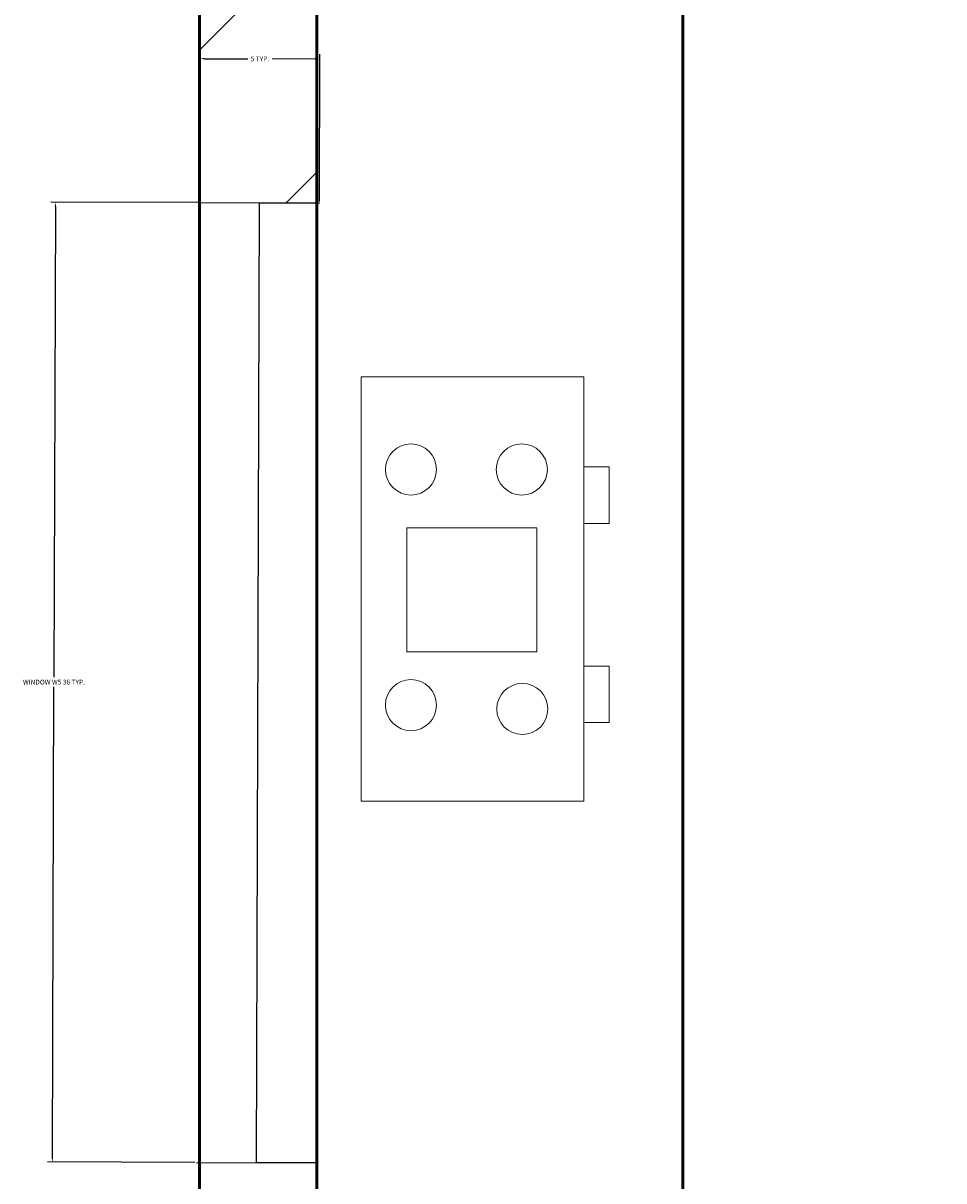
# Model space of a CAD drawing. Units: inches. Extents: x 1901 to 2863, y 888 to 2433.
# Tile 5 of 91: x 2018 to 2053, y 1466 to 1510. Entities that reach past the tile are written whole.
import ezdxf

# ---------------------------------------------------------------- set-up
doc = ezdxf.new("R2010")
doc.units = ezdxf.units.IN
for name, color, linetype, lineweight in [('A-ANNO-DIMS', 2, 'Continuous', 18), ('A-FLOR-FIXT', 9, 'Continuous', 18), ('A-GLAZ', 3, 'Continuous', 25), ('A-WALL', 7, 'Continuous', 50), ('A-WALL-PATT', 8, 'Continuous', 13)]:
    doc.layers.add(name, color=color, linetype=linetype, lineweight=lineweight)
doc.styles.get("Standard").update_dxf_attribs({"font": 'arial.ttf'})
doc.dimstyles.get("Standard").update_dxf_attribs({"dimtxt": 0.18, "dimasz": 0.18, "dimexe": 0.18, "dimexo": 0.0625, "dimgap": 0.09, "dimtad": 0, "dimtih": 1, "dimtoh": 1, "dimdec": 4, "dimzin": 0, "dimdsep": 46, "dimtxsty": 'Standard', "dimcen": 0.09, "dimadec": 0, "dimazin": 0, "dimtfac": 1, "dimtdec": 4, "dimtofl": 0, "dimtmove": 0, "dimatfit": 3, "dimfxl": 1, "dimtolj": 1, "dimtzin": 0, "dimarcsym": 0})

# ---------------------------------------------------------------- blocks, each defined once
blk = doc.blocks.new('WIN-36')
for p, q in [((4.5, 36), (0, 36)), ((0, 36), (2.25, 36)), ((2.25, 36), (2.25, 0)), ((2.25, 0), (0, 0)), ((0, 0), (4.5, 0))]:
    blk.add_line(p, q)
blk = doc.blocks.new('*D27')
at = {"layer": 'A-ANNO-DIMS', "color": 0, "lineweight": -2, "transparency": 16777216}
for p, q in [((2024.862, 1502.839), (2019.345, 1502.857)), ((2019.524, 1502.676), (2019.467, 1485.04)), ((2019.408, 1467.036), (2019.466, 1484.673)), ((2024.745, 1466.839), (2019.228, 1466.857))]:
    blk.add_line(p, q, dxfattribs=at)
at = {"layer": 'A-ANNO-DIMS', "color": 0, "transparency": 16777216}
for points in [[(2019.494, 1502.676), (2019.554, 1502.676), (2019.525, 1502.856)], [(2019.378, 1467.037), (2019.438, 1467.036), (2019.408, 1466.856)]]:
    blk.add_solid(points, dxfattribs=at)
at = {"layer": 'Defpoints', "color": 0, "transparency": 16777216}
for p in [(2024.925, 1502.839), (2019.408, 1466.856), (2024.807, 1466.839)]:
    blk.add_point(p, dxfattribs=at)
at = {"layer": 'A-ANNO-DIMS', "color": 0, "transparency": 16777216, "insert": (2019.466, 1484.856), "char_height": 0.18, "attachment_point": 5}
blk.add_mtext('\\A1;WINDOW W5 36 TYP.', dxfattribs=at)
blk = doc.blocks.new('*D28')
at = {"layer": 'A-ANNO-DIMS', "color": 0, "lineweight": -2, "transparency": 16777216}
for p, q in [((2024.925, 1502.901), (2024.943, 1508.419)), ((2025.123, 1508.238), (2026.734, 1508.233)), ((2029.262, 1508.224), (2027.651, 1508.23)), ((2029.425, 1502.886), (2029.443, 1508.404))]:
    blk.add_line(p, q, dxfattribs=at)
at = {"layer": 'A-ANNO-DIMS', "color": 0, "transparency": 16777216}
for points in [[(2025.123, 1508.268), (2025.122, 1508.208), (2024.943, 1508.239)], [(2029.263, 1508.254), (2029.262, 1508.194), (2029.442, 1508.224)]]:
    blk.add_solid(points, dxfattribs=at)
at = {"layer": 'Defpoints', "color": 0, "transparency": 16777216}
for p in [(2024.943, 1508.239), (2024.925, 1502.839), (2029.425, 1502.824)]:
    blk.add_point(p, dxfattribs=at)
at = {"layer": 'A-ANNO-DIMS', "color": 0, "transparency": 16777216, "insert": (2027.192, 1508.231), "char_height": 0.18, "attachment_point": 5}
blk.add_mtext('\\A1;5 TYP.', dxfattribs=at)

msp = doc.modelspace()

# ---------------------------------------------------------------- hatches: boundary and pattern name
at = {"layer": 'A-WALL-PATT'}
h = msp.add_hatch(dxfattribs=at)
h.set_pattern_fill('ANSI32', color=256)
h.paths.add_polyline_path([(2182.933, 1716.634), (2024.926, 1716.634), (2024.926, 1681.702), (2029.326, 1681.702), (2029.326, 1712.134), (2154.326, 1712.134), (2154.326, 1580.134), (2148.524, 1580.134), (2148.524, 1577.884), (2148.524, 1575.634), (2194.93, 1575.634), (2194.93, 1580.134), (2158.826, 1580.134), (2158.826, 1712.134), (2182.933, 1712.134)])
h.paths.add_polyline_path([(2301.069, 1716.634), (2242.933, 1716.634), (2242.933, 1712.134), (2283.826, 1712.134), (2283.826, 1685.535), (2288.326, 1685.535), (2288.326, 1712.134), (2301.069, 1712.134)])
h.paths.add_polyline_path([(2288.326, 1600.411), (2286.076, 1600.411), (2283.826, 1600.411), (2283.826, 1580.134), (2270.601, 1580.134), (2270.601, 1575.634), (2288.326, 1575.634)])
h.paths.add_polyline_path([(2295.926, 1953.634), (2271.447, 1953.634), (2271.447, 1949.134), (2291.426, 1949.134), (2291.426, 1941.244), (2295.926, 1941.244)])
h.paths.add_polyline_path([(2098.376, 1244.134), (2082.326, 1244.134), (2082.326, 1302.134), (2086.523, 1302.134), (2086.523, 1306.634), (2067.456, 1306.634), (2067.456, 1302.134), (2077.826, 1302.134), (2077.826, 1239.634), (2098.376, 1239.634), (2098.376, 1241.884)])
h.paths.add_polyline_path([(2217.308, 1306.634), (2158.826, 1306.634), (2158.826, 1451.634), (2162.716, 1451.634), (2162.716, 1453.884), (2162.716, 1456.134), (2154.326, 1456.134), (2154.326, 1443.134), (2151.91, 1443.134), (2151.91, 1438.634), (2154.326, 1438.634), (2154.326, 1306.634), (2109.307, 1306.634), (2109.307, 1304.384), (2109.307, 1302.134), (2154.326, 1302.134), (2154.326, 1244.134), (2122.376, 1244.134), (2122.376, 1239.634), (2154.326, 1239.634), (2154.326, 1223.634), (2163.326, 1223.634), (2181.008, 1223.634), (2181.008, 1225.884), (2181.008, 1228.134), (2163.326, 1228.134), (2163.326, 1258.222), (2158.826, 1258.222), (2158.826, 1302.134), (2217.308, 1302.134)])
h.paths.add_polyline_path([(2259.991, 1306.634), (2238.299, 1306.634), (2238.299, 1304.384), (2238.299, 1302.134), (2242.826, 1302.134), (2242.826, 1228.134), (2205.008, 1228.134), (2205.008, 1223.634), (2247.326, 1223.634), (2247.326, 1302.134), (2259.991, 1302.134), (2259.991, 1304.384)])
h.paths.add_polyline_path([(2343.426, 1361.697), (2338.926, 1361.697), (2338.926, 1306.634), (2322.38, 1306.634), (2322.38, 1302.134), (2343.426, 1302.134)])
h.paths.add_polyline_path([(2343.426, 1470.397), (2338.926, 1470.397), (2338.926, 1456.134), (2193.726, 1456.134), (2193.726, 1453.884), (2193.726, 1451.634), (2338.926, 1451.634), (2338.926, 1421.697), (2343.426, 1421.697)])
h.paths.add_polyline_path([(2343.426, 1545.507), (2338.926, 1545.507), (2338.926, 1530.397), (2343.426, 1530.397)])
h.paths.add_polyline_path([(2029.326, 1466.83), (2024.926, 1466.83), (2024.926, 1409.825), (2029.326, 1409.825)])
h.paths.add_polyline_path([(2122.843, 1440.884), (2122.843, 1443.134), (2121.826, 1443.134), (2121.826, 1498.183), (2119.576, 1498.183), (2117.326, 1498.183), (2117.326, 1443.134), (2029.326, 1443.134), (2029.326, 1438.634), (2122.843, 1438.634)])
h.paths.add_polyline_path([(2029.326, 1543.053), (2024.926, 1543.053), (2024.926, 1502.83), (2029.326, 1502.83)])
h.paths.add_polyline_path([(2029.326, 1621.702), (2024.926, 1621.702), (2024.926, 1567.053), (2027.126, 1567.053), (2029.326, 1567.053), (2029.326, 1575.634), (2109.326, 1575.634), (2109.326, 1554.715), (2113.826, 1554.715), (2113.826, 1575.634), (2115.805, 1575.634), (2115.805, 1577.884), (2115.805, 1580.134), (2029.326, 1580.134)])
h.paths.add_polyline_path([(2121.826, 1527.634), (2117.326, 1527.634), (2113.826, 1527.634), (2113.826, 1533.011), (2111.576, 1533.011), (2109.326, 1533.011), (2109.326, 1527.634), (2029.326, 1527.634), (2029.326, 1523.134), (2117.326, 1523.134), (2117.326, 1519.43), (2121.826, 1519.43)])
h.paths.add_polyline_path([(2029.326, 1349.825), (2024.926, 1349.825), (2024.926, 1302.134), (2036.277, 1302.134), (2036.277, 1306.634), (2029.326, 1306.634)])

# ---------------------------------------------------------------- linework, layer by layer
at = {"layer": 'A-FLOR-FIXT'}
for points in [[(2030.986, 1496.306), (2039.339, 1496.306), (2039.339, 1480.386), (2030.986, 1480.386)], [(2039.339, 1492.925), (2040.288, 1492.925), (2040.288, 1490.806), (2039.339, 1490.806)], [(2032.708, 1490.646), (2037.583, 1490.646), (2037.583, 1485.988), (2032.708, 1485.988)], [(2039.339, 1485.456), (2040.288, 1485.456), (2040.288, 1483.337), (2039.339, 1483.337)]]:
    msp.add_lwpolyline(points, close=True, dxfattribs=at)
for centre in [(2032.857, 1492.831), (2037.015, 1492.831), (2032.857, 1483.992), (2037.033, 1483.848)]:
    msp.add_circle(centre, 0.958, dxfattribs=at)
at = {"layer": 'A-WALL'}
for p, q in [((2024.926, 1716.634), (2024.926, 1302.134)), ((2029.326, 1575.634), (2029.326, 1306.634)), ((2043.059, 1456.597), (2043.059, 1523.134))]:
    msp.add_line(p, q, dxfattribs=at)

# ---------------------------------------------------------------- block references
at = {"layer": 'A-GLAZ', "rotation": 179.8131259740874}
msp.add_blockref('WIN-36', (2029.425, 1502.824), dxfattribs=at)

# ---------------------------------------------------------------- dimensions: what is measured, and where the dimension line sits
at = {"layer": 'A-ANNO-DIMS'}
for base, p1, p2, angle, text, picture, middle in [((2024.94251, 1508.23857), (2029.42487, 1502.82393), (2024.9249, 1502.8386), 179.81313, '<> TYP.', '*D28', (2027.1925, 1508.23124)), ((2019.408, 1466.856), (2024.925, 1502.839), (2024.807, 1466.839), 269.8131, 'WINDOW W5 <> TYP.', '*D27', (2019.466, 1484.856))]:
    dim = msp.add_linear_dim(base=base, p1=p1, p2=p2, angle=angle, text=text, dimstyle='Standard', override={"dimdec": 0, "dimlfac": 1, "dimrnd": 0, "dimzin": 0, "dimdsep": 46, "dimlunit": 2}, dxfattribs=at)
    dim.commit()
    dim.dimension.update_dxf_attribs({"geometry": picture, "text_midpoint": middle})

doc.saveas('drawing.dxf')
